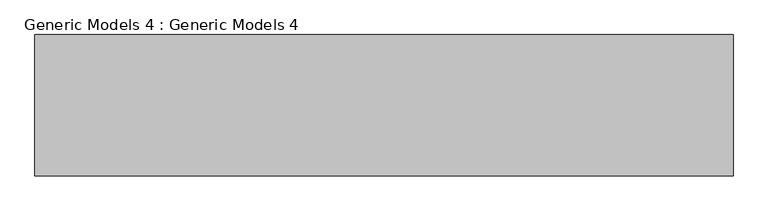
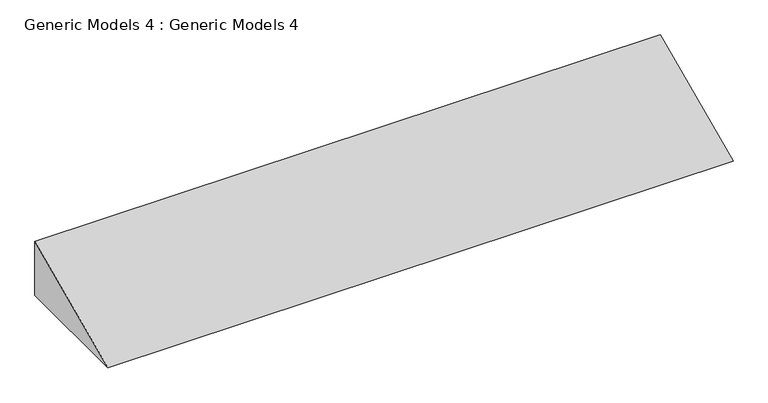
"""IFC4 building model written with IfcOpenShell, lengths in millimetres: proxy geometry, Generic Models 4 : Generic Models 4."""

from ifc_helpers import new_model, si_unit, frame, origin, place, context, project, spatial, polyline, outline, extrude, source, transform, mapped, element, save


def generic_models_4_generic_models_4_8b3ef071(model_context):
    return source(origin(), model_context, "Body", "SweptSolid", [
        extrude(outline(polyline([(-7265.2302427, 0.0), (-7830.3802427, 0.0), (-7265.2302427, 254.0), (-7265.2302427, 0.0)])), frame((-1012.4672301, 0.0, 0.0), z_axis=(1.0, 0.0, 0.0), x_axis=(0.0, 1.0, 0.0)), (0.0, 0.0, 1.0), 2794.0),
    ])


if __name__ == "__main__":
    model = new_model("IFC4")
    model_context = context("Model", 3, world=origin())
    ifc_project = project(units=[si_unit("LENGTHUNIT", "METRE", prefix="MILLI")], contexts=[model_context])
    site = spatial("IfcSite", under=ifc_project)
    building = spatial("IfcBuilding", under=site)
    placement = place(None, origin())
    generic_models_4_generic_models_4_shape = generic_models_4_generic_models_4_8b3ef071(model_context)
    element("IfcBuildingElementProxy", 1, Name="Generic Models 4 : Generic Models 4", ObjectType="Generic Models 4 : Generic Models 4", at=placement, inside=building, context=model_context, shape_type="MappedRepresentation", body=[
        mapped(generic_models_4_generic_models_4_shape, transform((0.0, 0.0, 0.0), x_axis=(1.0, 0.0, 0.0), y_axis=(0.0, 1.0, 0.0), z_axis=(0.0, 0.0, 1.0))),
    ])
    save(model, "model.ifc")

# Revit data of these elements
# Element 1 (IfcBuildingElementProxy, "Generic Models 4 : Generic Models 4")
#   Materials on its faces: "Laminate, Ivory, Matte"
# Materials
#   "Laminate, Ivory, Matte": class "Plastic", colour RGB 247 247 239, transparency 0, Description = "Plastic Laminate - Ivory, Matte", Cost = 0
